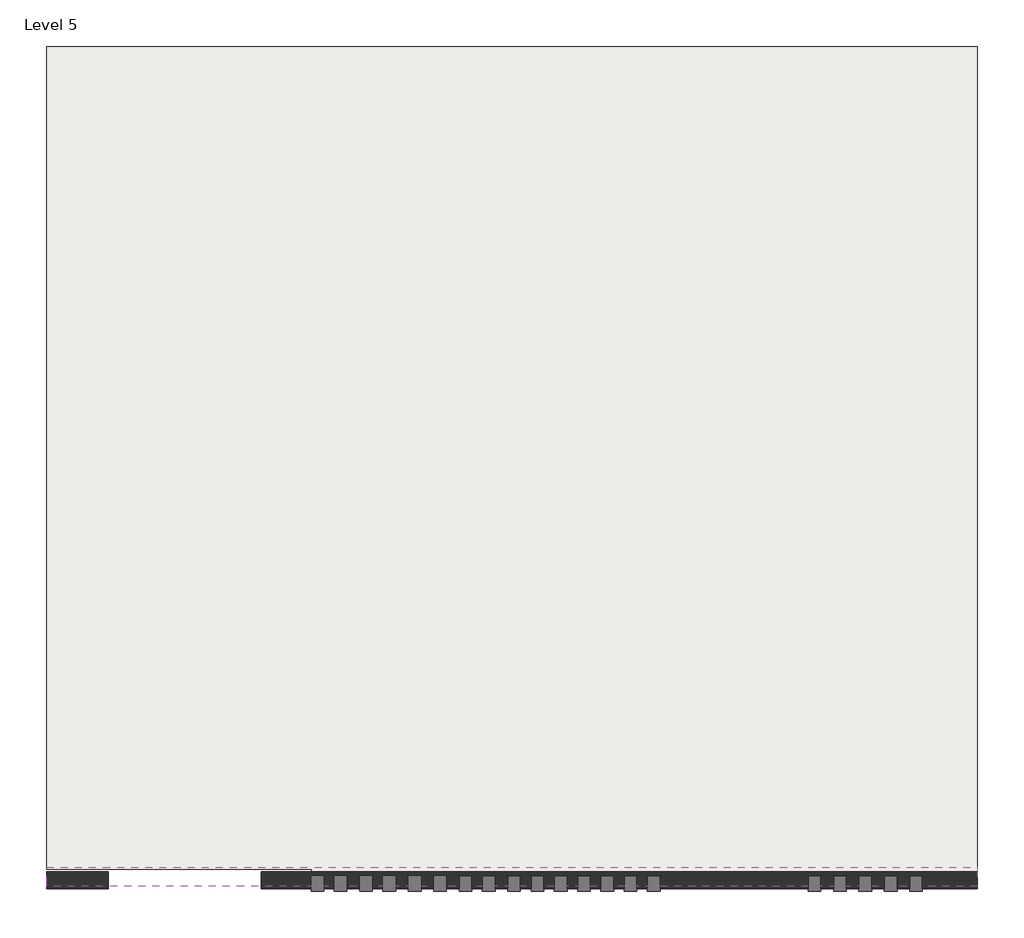
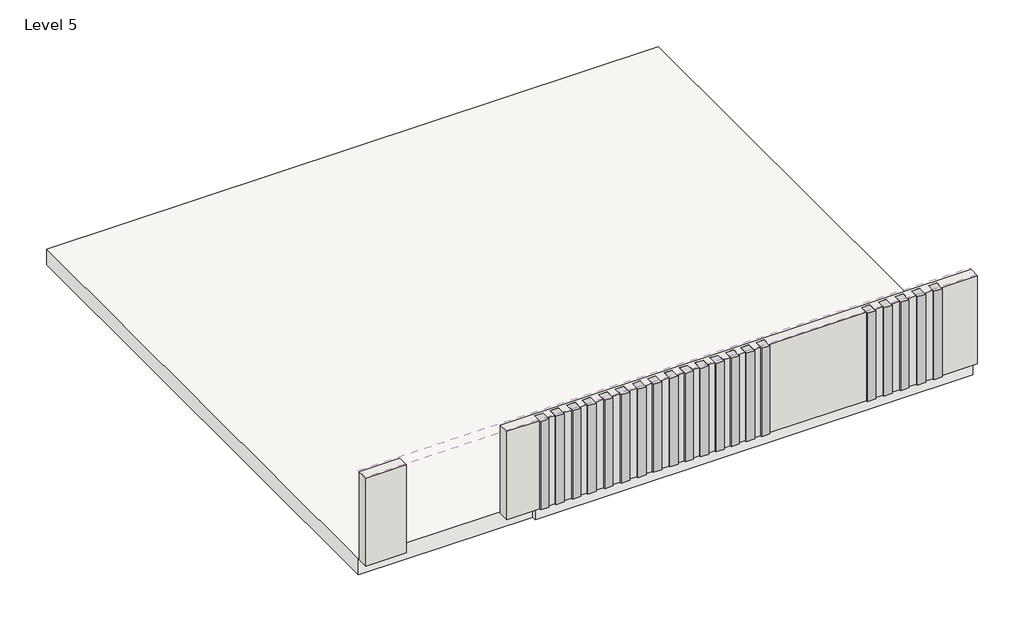
# One storey: 20 proxies, 2 roofs, 1 wall.
"""IFC4 building model written with IfcOpenShell, lengths in millimetres."""

from ifc_helpers import new_model, si_unit, frame, origin, place, context, project, spatial, polyline, outline, extrude, element, save

model = new_model("IFC4")

# Units and contexts
model_context = context("Model", 3, world=origin())
ifc_project = project(units=[si_unit("LENGTHUNIT", "METRE", prefix="MILLI")], contexts=[model_context])

# Site, building, storey
site = spatial("IfcSite", under=ifc_project)
building = spatial("IfcBuilding", under=site)
storey = spatial("IfcBuildingStorey", under=building, Name="Level 5", Elevation=14630.4)

# Proxies
placement = place(None, origin())
element("IfcBuildingElementProxy", 1, Name="Reveal", ObjectType="Reveal", at=placement, inside=storey, context=model_context, shape_type="SweptSolid", body=[
    extrude(outline(polyline([(-5851.4998814, 191.4810824), (-5851.4998814, 374.3610824), (-5699.0998814, 374.3610824), (-5699.0998814, 191.4810824), (-5851.4998814, 191.4810824)])), frame((0.0, 0.0, 14935.2), z_axis=(0.0, 0.0, 1.0), x_axis=(1.0, 0.0, 0.0)), (0.0, 0.0, 1.0), 1704.549675),
])
element("IfcBuildingElementProxy", 2, Name="Reveal", ObjectType="Reveal", at=placement, inside=storey, context=model_context, shape_type="SweptSolid", body=[
    extrude(outline(polyline([(-5572.0998814, 191.4810824), (-5572.0998814, 374.3610824), (-5419.6998814, 374.3610824), (-5419.6998814, 191.4810824), (-5572.0998814, 191.4810824)])), frame((0.0, 0.0, 14935.2), z_axis=(0.0, 0.0, 1.0), x_axis=(1.0, 0.0, 0.0)), (0.0, 0.0, 1.0), 1704.549675),
])
element("IfcBuildingElementProxy", 3, Name="Reveal", ObjectType="Reveal", at=placement, inside=storey, context=model_context, shape_type="SweptSolid", body=[
    extrude(outline(polyline([(-5267.2998814, 191.4810824), (-5267.2998814, 374.3610824), (-5114.8998814, 374.3610824), (-5114.8998814, 191.4810824), (-5267.2998814, 191.4810824)])), frame((0.0, 0.0, 14935.2), z_axis=(0.0, 0.0, 1.0), x_axis=(1.0, 0.0, 0.0)), (0.0, 0.0, 1.0), 1704.549675),
])
element("IfcBuildingElementProxy", 4, Name="Reveal", ObjectType="Reveal", at=placement, inside=storey, context=model_context, shape_type="SweptSolid", body=[
    extrude(outline(polyline([(-4987.8998814, 191.4810824), (-4987.8998814, 374.3610824), (-4835.4998814, 374.3610824), (-4835.4998814, 191.4810824), (-4987.8998814, 191.4810824)])), frame((0.0, 0.0, 14935.2), z_axis=(0.0, 0.0, 1.0), x_axis=(1.0, 0.0, 0.0)), (0.0, 0.0, 1.0), 1704.549675),
])
element("IfcBuildingElementProxy", 5, Name="Reveal", ObjectType="Reveal", at=placement, inside=storey, context=model_context, shape_type="SweptSolid", body=[
    extrude(outline(polyline([(-4683.0998814, 191.4810824), (-4683.0998814, 374.3610824), (-4530.6998814, 374.3610824), (-4530.6998814, 191.4810824), (-4683.0998814, 191.4810824)])), frame((0.0, 0.0, 14935.2), z_axis=(0.0, 0.0, 1.0), x_axis=(1.0, 0.0, 0.0)), (0.0, 0.0, 1.0), 1704.549675),
])
element("IfcBuildingElementProxy", 6, Name="Reveal", ObjectType="Reveal", at=placement, inside=storey, context=model_context, shape_type="SweptSolid", body=[
    extrude(outline(polyline([(-4378.2998814, 191.4810824), (-4378.2998814, 374.3610824), (-4225.8998814, 374.3610824), (-4225.8998814, 191.4810824), (-4378.2998814, 191.4810824)])), frame((0.0, 0.0, 14935.2), z_axis=(0.0, 0.0, 1.0), x_axis=(1.0, 0.0, 0.0)), (0.0, 0.0, 1.0), 1704.549675),
])
element("IfcBuildingElementProxy", 7, Name="Reveal", ObjectType="Reveal", at=placement, inside=storey, context=model_context, shape_type="SweptSolid", body=[
    extrude(outline(polyline([(-4073.4998814, 191.4810824), (-4073.4998814, 374.3610824), (-3921.0998814, 374.3610824), (-3921.0998814, 191.4810824), (-4073.4998814, 191.4810824)])), frame((0.0, 0.0, 14935.2), z_axis=(0.0, 0.0, 1.0), x_axis=(1.0, 0.0, 0.0)), (0.0, 0.0, 1.0), 1704.549675),
])
element("IfcBuildingElementProxy", 8, Name="Reveal", ObjectType="Reveal", at=placement, inside=storey, context=model_context, shape_type="SweptSolid", body=[
    extrude(outline(polyline([(-3794.0998814, 191.4810824), (-3794.0998814, 374.3610824), (-3641.6998814, 374.3610824), (-3641.6998814, 191.4810824), (-3794.0998814, 191.4810824)])), frame((0.0, 0.0, 14935.2), z_axis=(0.0, 0.0, 1.0), x_axis=(1.0, 0.0, 0.0)), (0.0, 0.0, 1.0), 1704.549675),
])
element("IfcBuildingElementProxy", 9, Name="Reveal", ObjectType="Reveal", at=placement, inside=storey, context=model_context, shape_type="SweptSolid", body=[
    extrude(outline(polyline([(-3489.2998814, 191.4810824), (-3489.2998814, 374.3610824), (-3336.8998814, 374.3610824), (-3336.8998814, 191.4810824), (-3489.2998814, 191.4810824)])), frame((0.0, 0.0, 14935.2), z_axis=(0.0, 0.0, 1.0), x_axis=(1.0, 0.0, 0.0)), (0.0, 0.0, 1.0), 1704.549675),
])
element("IfcBuildingElementProxy", 10, Name="Reveal", ObjectType="Reveal", at=placement, inside=storey, context=model_context, shape_type="SweptSolid", body=[
    extrude(outline(polyline([(-3209.8998814, 191.4810824), (-3209.8998814, 374.3610824), (-3057.4998814, 374.3610824), (-3057.4998814, 191.4810824), (-3209.8998814, 191.4810824)])), frame((0.0, 0.0, 14935.2), z_axis=(0.0, 0.0, 1.0), x_axis=(1.0, 0.0, 0.0)), (0.0, 0.0, 1.0), 1704.549675),
])
element("IfcBuildingElementProxy", 11, Name="Reveal", ObjectType="Reveal", at=placement, inside=storey, context=model_context, shape_type="SweptSolid", body=[
    extrude(outline(polyline([(-2930.4998814, 191.4810824), (-2930.4998814, 374.3610824), (-2778.0998814, 374.3610824), (-2778.0998814, 191.4810824), (-2930.4998814, 191.4810824)])), frame((0.0, 0.0, 14935.2), z_axis=(0.0, 0.0, 1.0), x_axis=(1.0, 0.0, 0.0)), (0.0, 0.0, 1.0), 1704.549675),
])
element("IfcBuildingElementProxy", 12, Name="Reveal", ObjectType="Reveal", at=placement, inside=storey, context=model_context, shape_type="SweptSolid", body=[
    extrude(outline(polyline([(-2651.0998814, 191.4810824), (-2651.0998814, 374.3610824), (-2498.6998814, 374.3610824), (-2498.6998814, 191.4810824), (-2651.0998814, 191.4810824)])), frame((0.0, 0.0, 14935.2), z_axis=(0.0, 0.0, 1.0), x_axis=(1.0, 0.0, 0.0)), (0.0, 0.0, 1.0), 1704.549675),
])
element("IfcBuildingElementProxy", 13, Name="Reveal", ObjectType="Reveal", at=placement, inside=storey, context=model_context, shape_type="SweptSolid", body=[
    extrude(outline(polyline([(-2371.6998814, 191.4810824), (-2371.6998814, 374.3610824), (-2219.2998814, 374.3610824), (-2219.2998814, 191.4810824), (-2371.6998814, 191.4810824)])), frame((0.0, 0.0, 14935.2), z_axis=(0.0, 0.0, 1.0), x_axis=(1.0, 0.0, 0.0)), (0.0, 0.0, 1.0), 1704.549675),
])
element("IfcBuildingElementProxy", 14, Name="Reveal", ObjectType="Reveal", at=placement, inside=storey, context=model_context, shape_type="SweptSolid", body=[
    extrude(outline(polyline([(-2092.2998814, 191.4810824), (-2092.2998814, 374.3610824), (-1939.8998814, 374.3610824), (-1939.8998814, 191.4810824), (-2092.2998814, 191.4810824)])), frame((0.0, 0.0, 14935.2), z_axis=(0.0, 0.0, 1.0), x_axis=(1.0, 0.0, 0.0)), (0.0, 0.0, 1.0), 1704.549675),
])
element("IfcBuildingElementProxy", 15, Name="Reveal", ObjectType="Reveal", at=placement, inside=storey, context=model_context, shape_type="SweptSolid", body=[
    extrude(outline(polyline([(-1812.8998814, 191.4810824), (-1812.8998814, 374.3610824), (-1660.4998814, 374.3610824), (-1660.4998814, 191.4810824), (-1812.8998814, 191.4810824)])), frame((0.0, 0.0, 14935.2), z_axis=(0.0, 0.0, 1.0), x_axis=(1.0, 0.0, 0.0)), (0.0, 0.0, 1.0), 1704.549675),
])
element("IfcBuildingElementProxy", 16, Name="Reveal", ObjectType="Reveal", at=placement, inside=storey, context=model_context, shape_type="SweptSolid", body=[
    extrude(outline(polyline([(117.5001186, 191.4810824), (117.5001186, 374.3610824), (269.9001186, 374.3610824), (269.9001186, 191.4810824), (117.5001186, 191.4810824)])), frame((0.0, 0.0, 14935.2), z_axis=(0.0, 0.0, 1.0), x_axis=(1.0, 0.0, 0.0)), (0.0, 0.0, 1.0), 1704.549675),
])
element("IfcBuildingElementProxy", 17, Name="Reveal", ObjectType="Reveal", at=placement, inside=storey, context=model_context, shape_type="SweptSolid", body=[
    extrude(outline(polyline([(422.3001186, 191.4810824), (422.3001186, 374.3610824), (574.7001186, 374.3610824), (574.7001186, 191.4810824), (422.3001186, 191.4810824)])), frame((0.0, 0.0, 14935.2), z_axis=(0.0, 0.0, 1.0), x_axis=(1.0, 0.0, 0.0)), (0.0, 0.0, 1.0), 1704.549675),
])
element("IfcBuildingElementProxy", 18, Name="Reveal", ObjectType="Reveal", at=placement, inside=storey, context=model_context, shape_type="SweptSolid", body=[
    extrude(outline(polyline([(727.1001186, 191.4810824), (727.1001186, 374.3610824), (879.5001186, 374.3610824), (879.5001186, 191.4810824), (727.1001186, 191.4810824)])), frame((0.0, 0.0, 14935.2), z_axis=(0.0, 0.0, 1.0), x_axis=(1.0, 0.0, 0.0)), (0.0, 0.0, 1.0), 1704.549675),
])
element("IfcBuildingElementProxy", 19, Name="Reveal", ObjectType="Reveal", at=placement, inside=storey, context=model_context, shape_type="SweptSolid", body=[
    extrude(outline(polyline([(1031.9001186, 191.4810824), (1031.9001186, 374.3610824), (1184.3001186, 374.3610824), (1184.3001186, 191.4810824), (1031.9001186, 191.4810824)])), frame((0.0, 0.0, 14935.2), z_axis=(0.0, 0.0, 1.0), x_axis=(1.0, 0.0, 0.0)), (0.0, 0.0, 1.0), 1704.549675),
])
element("IfcBuildingElementProxy", 20, Name="Reveal", ObjectType="Reveal", at=placement, inside=storey, context=model_context, shape_type="SweptSolid", body=[
    extrude(outline(polyline([(1336.7001186, 191.4810824), (1336.7001186, 374.3610824), (1489.1001186, 374.3610824), (1489.1001186, 191.4810824), (1336.7001186, 191.4810824)])), frame((0.0, 0.0, 14935.2), z_axis=(0.0, 0.0, 1.0), x_axis=(1.0, 0.0, 0.0)), (0.0, 0.0, 1.0), 1704.549675),
])

# Roofs
element("IfcRoof", 21, ObjectType="Generic - 12\"", at=placement, inside=storey, context=model_context, shape_type="SweptSolid", body=[
    extrude(outline(polyline([(-9026.4998814, 10331.1610824), (2149.5001186, 10331.1610824), (2149.5001186, 374.3610824), (-5845.1498814, 374.3610824), (-5845.1498814, 456.9110824), (-9026.4998814, 456.9110824), (-9026.4998814, 10331.1610824)])), frame((0.0, 0.0, 14630.4), z_axis=(0.0, 0.0, 1.0), x_axis=(1.0, 0.0, 0.0)), (0.0, 0.0, 1.0), 304.8),
])
element("IfcRoof", 22, ObjectType="Generic - 12\"", at=placement, inside=storey, context=model_context, shape_type="SweptSolid", body=[
    extrude(outline(polyline([(-9026.4998814, 475.9610824), (2149.5001186, 475.9610824), (2149.5001186, 247.3610824), (-9026.4998814, 247.3610824), (-9026.4998814, 475.9610824)])), frame((0.0, 0.0, 16637.0), z_axis=(0.0, 0.0, 1.0), x_axis=(1.0, 0.0, 0.0)), (0.0, 0.0, 1.0), 304.8),
])

# Wall
element("IfcWall", 23, ObjectType="Generic - 8\"", at=placement, inside=storey, context=model_context, shape_type="SweptSolid", body=[
    extrude(outline(polyline([(-6450.1094885, 425.1610824), (2149.5001186, 425.1610824), (2149.5001186, 221.9610824), (1489.1001186, 221.9610824), (1489.1001186, 374.3610824), (1336.7001186, 374.3610824), (1336.7001186, 221.9610824), (1184.3001186, 221.9610824), (1184.3001186, 374.3610824), (1031.9001186, 374.3610824), (1031.9001186, 221.9610824), (879.5001186, 221.9610824), (879.5001186, 374.3610824), (727.1001186, 374.3610824), (727.1001186, 221.9610824), (574.7001186, 221.9610824), (574.7001186, 374.3610824), (422.3001186, 374.3610824), (422.3001186, 221.9610824), (269.9001186, 221.9610824), (269.9001186, 374.3610824), (117.5001186, 374.3610824), (117.5001186, 221.9610824), (-1660.4998814, 221.9610824), (-1660.4998814, 374.3610824), (-1812.8998814, 374.3610824), (-1812.8998814, 221.9610824), (-1939.8998814, 221.9610824), (-1939.8998814, 374.3610824), (-2092.2998814, 374.3610824), (-2092.2998814, 221.9610824), (-2219.2998814, 221.9610824), (-2219.2998814, 374.3610824), (-2371.6998814, 374.3610824), (-2371.6998814, 221.9610824), (-2498.6998814, 221.9610824), (-2498.6998814, 374.3610824), (-2651.0998814, 374.3610824), (-2651.0998814, 221.9610824), (-2778.0998814, 221.9610824), (-2778.0998814, 374.3610824), (-2930.4998814, 374.3610824), (-2930.4998814, 221.9610824), (-3057.4998814, 221.9610824), (-3057.4998814, 374.3610824), (-3209.8998814, 374.3610824), (-3209.8998814, 221.9610824), (-3336.8998814, 221.9610824), (-3336.8998814, 374.3610824), (-3489.2998814, 374.3610824), (-3489.2998814, 221.9610824), (-3641.6998814, 221.9610824), (-3641.6998814, 374.3610824), (-3794.0998814, 374.3610824), (-3794.0998814, 221.9610824), (-3921.0998814, 221.9610824), (-3921.0998814, 374.3610824), (-4073.4998814, 374.3610824), (-4073.4998814, 221.9610824), (-4225.8998814, 221.9610824), (-4225.8998814, 374.3610824), (-4378.2998814, 374.3610824), (-4378.2998814, 221.9610824), (-4530.6998814, 221.9610824), (-4530.6998814, 374.3610824), (-4683.0998814, 374.3610824), (-4683.0998814, 221.9610824), (-4835.4998814, 221.9610824), (-4835.4998814, 374.3610824), (-4987.8998814, 374.3610824), (-4987.8998814, 221.9610824), (-5114.8998814, 221.9610824), (-5114.8998814, 374.3610824), (-5267.2998814, 374.3610824), (-5267.2998814, 221.9610824), (-5419.6998814, 221.9610824), (-5419.6998814, 374.3610824), (-5572.0998814, 374.3610824), (-5572.0998814, 221.9610824), (-5699.0998814, 221.9610824), (-5699.0998814, 374.3610824), (-5851.4998814, 374.3610824), (-5851.4998814, 221.9610824), (-6450.1094885, 221.9610824), (-6450.1094885, 425.1610824)])), frame((0.0, 0.0, 14935.2), z_axis=(0.0, 0.0, 1.0), x_axis=(1.0, 0.0, 0.0)), (0.0, 0.0, 1.0), 1704.549675),
    extrude(outline(polyline([(-8287.9658506, 221.9610824), (-9026.4998814, 221.9610824), (-9026.4998814, 425.1610824), (-8287.9658506, 425.1610824), (-8287.9658506, 221.9610824)])), frame((0.0, 0.0, 14935.2), z_axis=(0.0, 0.0, 1.0), x_axis=(1.0, 0.0, 0.0)), (0.0, 0.0, 1.0), 1704.549675),
])

save(model, "model.ifc")

# Revit data of these elements
# Type "Generic - 12\""
#   Assembly Code = "B1020"
#   Layers, outside or top first: 1' - 0" no material (function 1)
# Type "Generic - 8\""
#   Assembly Code = "B2010"
#   Layers, outside or top first: 0' - 8" no material (function 1)
# Element 21 (IfcRoof, "Generic - 12\"")
#   built-in parameter 1001705 = 49 (stored number, unit not read)
#   built-in parameter 1001710 = 33615
#   Phase Created = New Construction
#   Materials on its faces: "Default Roof"
# Element 22 (IfcRoof, "Generic - 12\"")
#   built-in parameter 1001705 = 55.5833 (stored number, unit not read)
#   built-in parameter 1001701 = 6.58333 (stored number, unit not read)
#   built-in parameter 1001710 = 33615
#   Phase Created = New Construction
#   Materials on its faces: "Default Roof"
# Element 23 (IfcWall, "Generic - 8\"")
#   built-in parameter 1001111 = 1' - 0"
#   Top Offset = 0' - 0"
#   Base Offset = 1' - 0"
#   Unconnected Height = 5' - 7.10825"
#   wall height = 5' - 7.10825"
#   Phase Created = New Construction
#   Base Constraint = Level 5
#   Materials on its faces: "Default Wall"
# Materials
#   "Default Roof": colour RGB 88 101 114, transparency 0
#   "Default Wall": colour RGB 128 128 128, transparency 0
